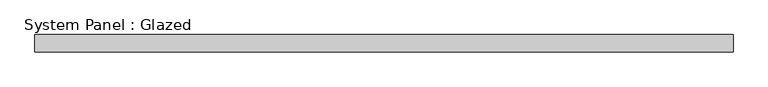
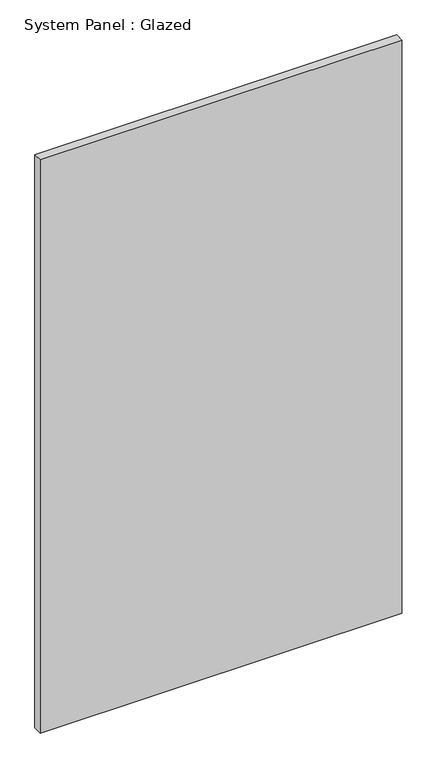
"""IFC4 building model written with IfcOpenShell, lengths in millimetres: plate geometry, System Panel : Glazed."""

from ifc_helpers import new_model, si_unit, origin, origin_with_axes, place, context, project, spatial, polyline, outline, extrude, source, transform, mapped, element, save


def system_panel_glazed_e830b44b(model_context):
    return source(origin(), model_context, "Body", "SweptSolid", [
        extrude(outline(polyline([(508.0, 19.05), (-508.0, 19.05), (-508.0, 44.45), (508.0, 44.45), (508.0, 19.05)])), origin_with_axes(), (0.0, 0.0, 1.0), 1701.8),
    ])


if __name__ == "__main__":
    model = new_model("IFC4")
    model_context = context("Model", 3, world=origin())
    ifc_project = project(units=[si_unit("LENGTHUNIT", "METRE", prefix="MILLI")], contexts=[model_context])
    site = spatial("IfcSite", under=ifc_project)
    building = spatial("IfcBuilding", under=site)
    placement = place(None, origin())
    system_panel_glazed_shape = system_panel_glazed_e830b44b(model_context)
    element("IfcPlate", 1, ObjectType="System Panel : Glazed", at=placement, inside=building, context=model_context, shape_type="MappedRepresentation", body=[
        mapped(system_panel_glazed_shape, transform((0.0, 0.0, 0.0), x_axis=(1.0, 0.0, 0.0), y_axis=(0.0, 1.0, 0.0), z_axis=(0.0, 0.0, 1.0))),
    ])
    save(model, "model.ifc")

# Revit data of these elements
# Type "System Panel : Glazed"
#   Construction Type Id = "GSP4R"
#   Analytic Construction = "1/8 in Pilkington single glazing"
#   Visual Light Transmittance = 0.9
#   Solar Heat Gain Coefficient = 0.86
#   Heat Transfer Coefficient (U) = 1.18115 BTU/(h·ft²·°F)
# Element 1 (IfcPlate, "System Panel : Glazed")
#   Materials on its faces: "Glass"
# Materials
#   "Glass": class "Glass", colour RGB 0 128 192, transparency 0.75, Description = "Soda Lime Glass", Cost = 0
